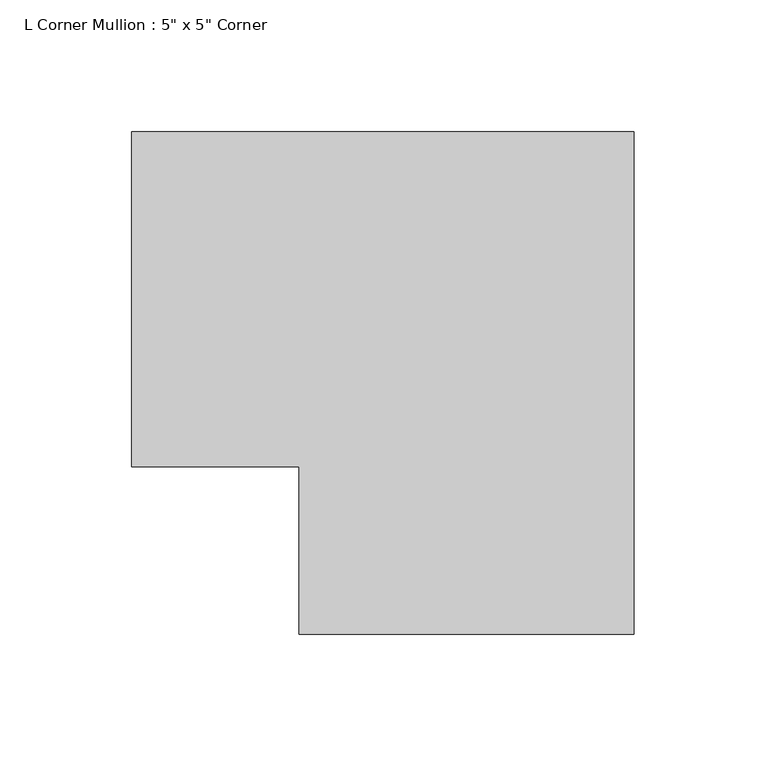
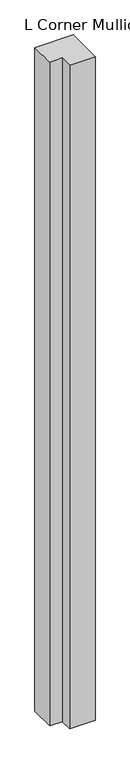
"""IFC4 building model written with IfcOpenShell, lengths in millimetres: member geometry."""

from ifc_helpers import new_model, si_unit, frame, origin, place, context, project, spatial, polyline, outline, extrude, source, transform, mapped, element, save


def member_693e8272(model_context):
    return source(origin(), model_context, "Body", "SweptSolid", [
        extrude(outline(polyline([(-63.5, -127.0), (-63.5, -63.5), (-127.0, -63.5), (-127.0, 63.5), (63.5, 63.5), (63.5, -127.0), (-63.5, -127.0)])), frame((0.0, 0.0, -3506.9820397), z_axis=(0.0, 0.0, 1.0), x_axis=(1.0, 0.0, 0.0)), (0.0, 0.0, 1.0), 3506.9820397),
    ])


if __name__ == "__main__":
    model = new_model("IFC4")
    model_context = context("Model", 3, world=origin())
    ifc_project = project(units=[si_unit("LENGTHUNIT", "METRE", prefix="MILLI")], contexts=[model_context])
    site = spatial("IfcSite", under=ifc_project)
    building = spatial("IfcBuilding", under=site)
    placement = place(None, origin())
    member_shape = member_693e8272(model_context)
    element("IfcMember", 1, ObjectType="L Corner Mullion : 5\" x 5\" Corner", at=placement, inside=building, context=model_context, shape_type="MappedRepresentation", body=[
        mapped(member_shape, transform((0.0, 0.0, 0.0), x_axis=(1.0, 0.0, 0.0), y_axis=(0.0, 1.0, 0.0), z_axis=(0.0, 0.0, 1.0))),
    ])
    save(model, "model.ifc")

# Revit data of these elements
# Type "L Corner Mullion : 5\" x 5\" Corner"
#   built-in parameter 1007355 = 0.416667 (stored number, unit not read)
#   built-in parameter 1007354 = 0.416667 (stored number, unit not read)
#   built-in parameter 1007304 = 0.416667 (stored number, unit not read)
# Element 1 (IfcMember, "L Corner Mullion : 5\" x 5\" Corner")
#   Materials on its faces: "Damp-proofing"
# Materials
#   "Damp-proofing": class "Generic", colour RGB 127 127 127, transparency 0, Description = "Damp-proofing", Cost = 0
